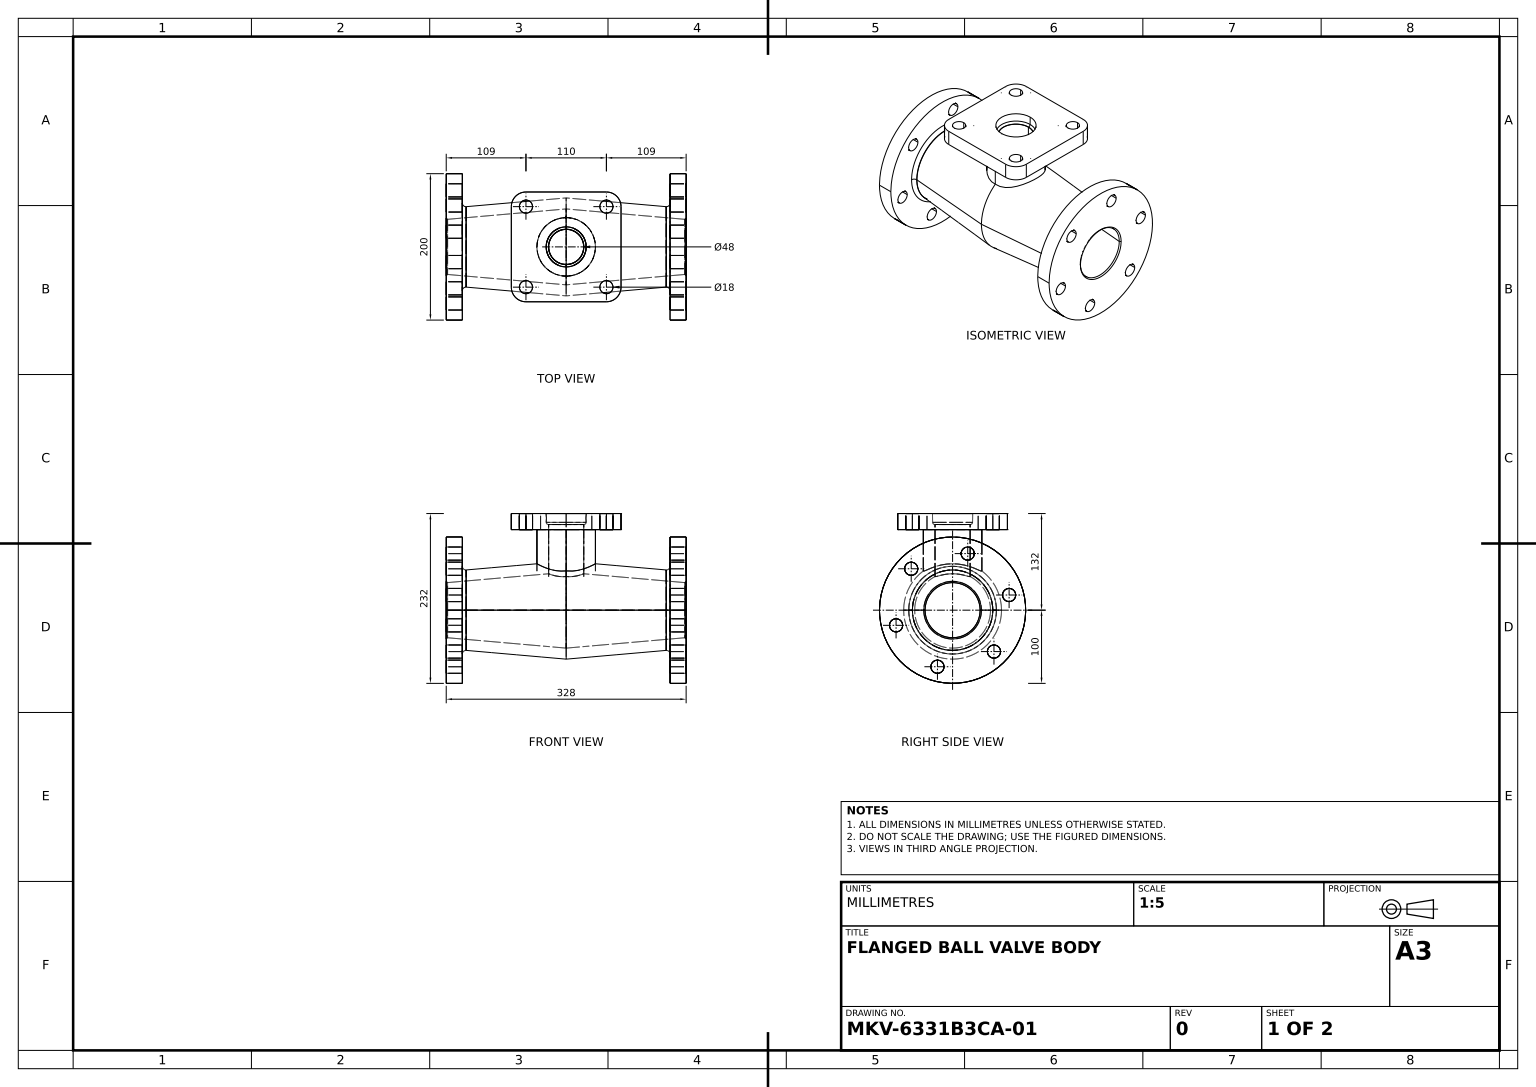
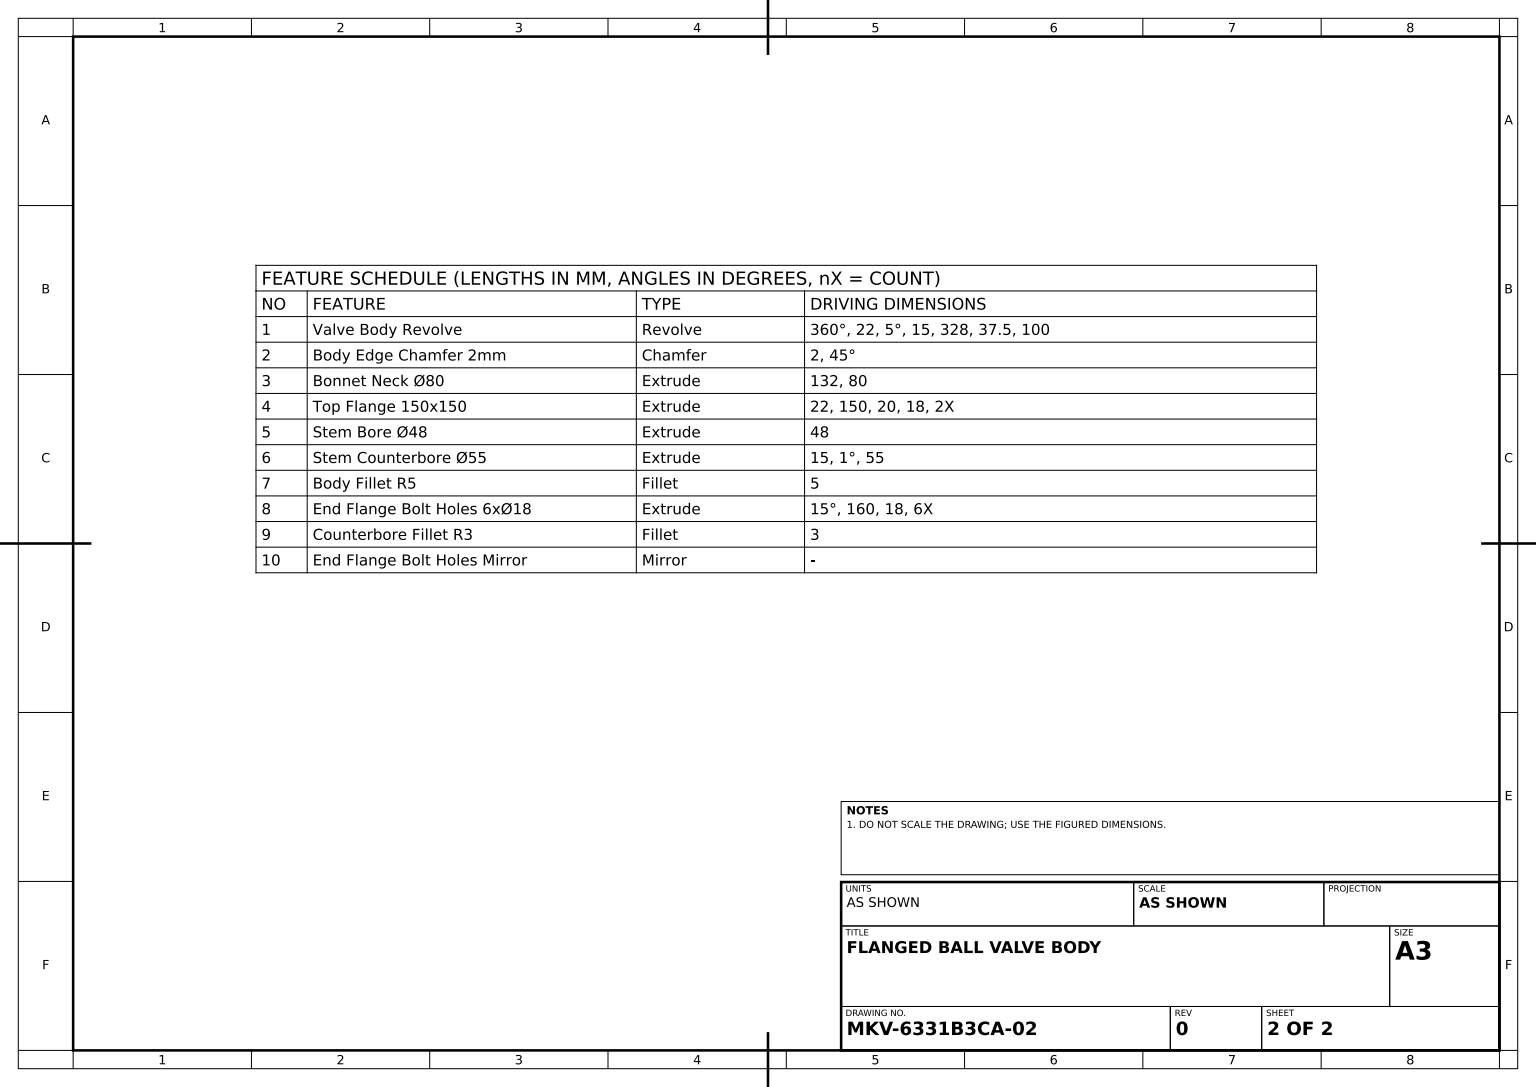
SolidWorks part; units mm, degrees
material "Plain Carbon Steel"
ref_plane "Front Plane" through (0, 0, 0) normal (0, 0, 1) x (1, 0, 0)
ref_plane "Top Plane" through (0, 0, 0) normal (0, 1, 0) x (1, 0, 0)
ref_plane "Right Plane" through (0, 0, 0) normal (1, 0, 0) x (0, 0, -1)
sketch "Body Profile Sketch" plane through (0, 0, 0) normal (0, 0, 1) x (1, 0, 0)
  line L0 (-175.4762, 0) -> (203.7619, 0) construction
  line L1 (-142, -54.482) -> (0, -66.9054)
  line L2 (0, -66.9054) -> (142, -54.482)
  line L3 (142, -54.482) -> (142, -100)
  line L4 (142, -100) -> (164, -100)
  line L5 (164, -100) -> (164, -37.5)
  line L6 (164, -37.5) -> (0, -51.8481)
  line L7 (0, -51.8481) -> (-164, -37.5)
  line L8 (-164, -37.5) -> (-164, -100)
  line L9 (-164, -100) -> (-142, -100)
  line L10 (-142, -100) -> (-142, -54.482)
  dimension "D1" = 22
  dimension "D2" = 37.5
  dimension "D3" = 5
  dimension "D4" = 5
  dimension "D5" = 15
  dimension "D6" = 328
  dimension "D7" = 100
revolve "Valve Body Revolve" add sketch "Body Profile Sketch" angle 360 about L0
chamfer "Body Edge Chamfer 2mm" distance 2 angle 45 2 edges at (164, 0, 37.5) (-164, 0, 37.5)
ref_plane "Plane2" through (0, 132, 0) normal (0, 1, 0) x (1, 0, 0)
sketch "Bonnet Neck Sketch" plane through (0, 132, 0) normal (0, 1, 0) x (1, 0, 0)
  circle A0 centre (0, 0) radius 40
  dimension "D1" = 80
extrude "Bonnet Neck Ø80" add sketch "Bonnet Neck Sketch" against normal up to surface (99.0116 mm away)
sketch "Top Flange Sketch" plane through (0, 132, 0) normal (0, 1, 0) x (1, 0, 0)
  line L1 (-55, -75) -> (55, -75)
  line L2 (-75, -55) -> (-75, 55)
  line L3 (-55, 75) -> (55, 75)
  line L4 (75, -55) -> (75, 55)
  line L5 (-75, -75) -> (75, 75) construction
  line L6 (-75, 75) -> (75, -75) construction
  arc A0 (-75, -55) -> (-55, -75) centre (-55, -55) ccw
  arc A1 (55, -75) -> (75, -55) centre (55, -55) ccw
  arc A2 (75, 55) -> (55, 75) centre (55, 55) ccw
  arc A3 (-55, 75) -> (-75, 55) centre (-55, 55) ccw
  circle A4 centre (-55, 55) radius 9
  circle A5 centre (55, 55) radius 9
  circle A6 centre (55, -55) radius 9
  circle A7 centre (-55, -55) radius 9
  point P0 (0, 0)
  dimension "D3" = 20
  dimension "D4" = 18
  dimension "D1" = 150
  dimension "D2" = 150
  dimension "D5" = 2
  dimension "D6" = 2
extrude "Top Flange 150x150" add sketch "Top Flange Sketch" against normal blind 22
sketch "Stem Bore Sketch" plane through (0, 132, 0) normal (0, 1, 0) x (1, 0, 0)
  circle A0 centre (0, 0) radius 24
  dimension "D1" = 48
extrude "Stem Bore Ø48" cut sketch "Stem Bore Sketch" against normal up to next
sketch "Stem Counterbore Sketch" plane through (0, 132, 0) normal (0, 1, 0) x (1, 0, 0)
  circle A0 centre (0, 0) radius 27.5
  dimension "D1" = 55
extrude "Stem Counterbore Ø55" cut sketch "Stem Counterbore Sketch" against normal blind 15 draft 1
fillet "Body Fillet R5" radius 5 2 edges at (142, 0, 54.482) (-142, 0, 54.482)
sketch "End Flange Bolt Holes Sketch" plane through (164, 0, 0) normal (1, 0, 0) x (0, 0, -1)
  line L0 (0, 0) -> (-126.2301, -33.8233) construction
  line L1 (0, 0) -> (-177.9947, 0) construction
  line L2 (0, 0) -> (0, -137.4197) construction
  circle A0 centre (0, 0) radius 80 construction
  circle A1 centre (-77.2741, -20.7055) radius 9
  circle A2 centre (-56.5685, 56.5685) radius 9
  circle A3 centre (20.7055, 77.2741) radius 9
  circle A4 centre (77.2741, 20.7055) radius 9
  circle A5 centre (56.5685, -56.5685) radius 9
  circle A6 centre (-20.7055, -77.2741) radius 9
  dimension "D2" = 160
  dimension "D3" = 18
  dimension "D1" = 15
  dimension "D4" = 6
extrude "End Flange Bolt Holes 6xØ18" cut sketch "End Flange Bolt Holes Sketch" against normal up to next
fillet "Counterbore Fillet R3" radius 3 1 edges at (0, 117, 27.2382)
mirror "End Flange Bolt Holes Mirror" about plane through (0, 0, 0) normal (1, 0, 0) of "End Flange Bolt Holes 6xØ18"
